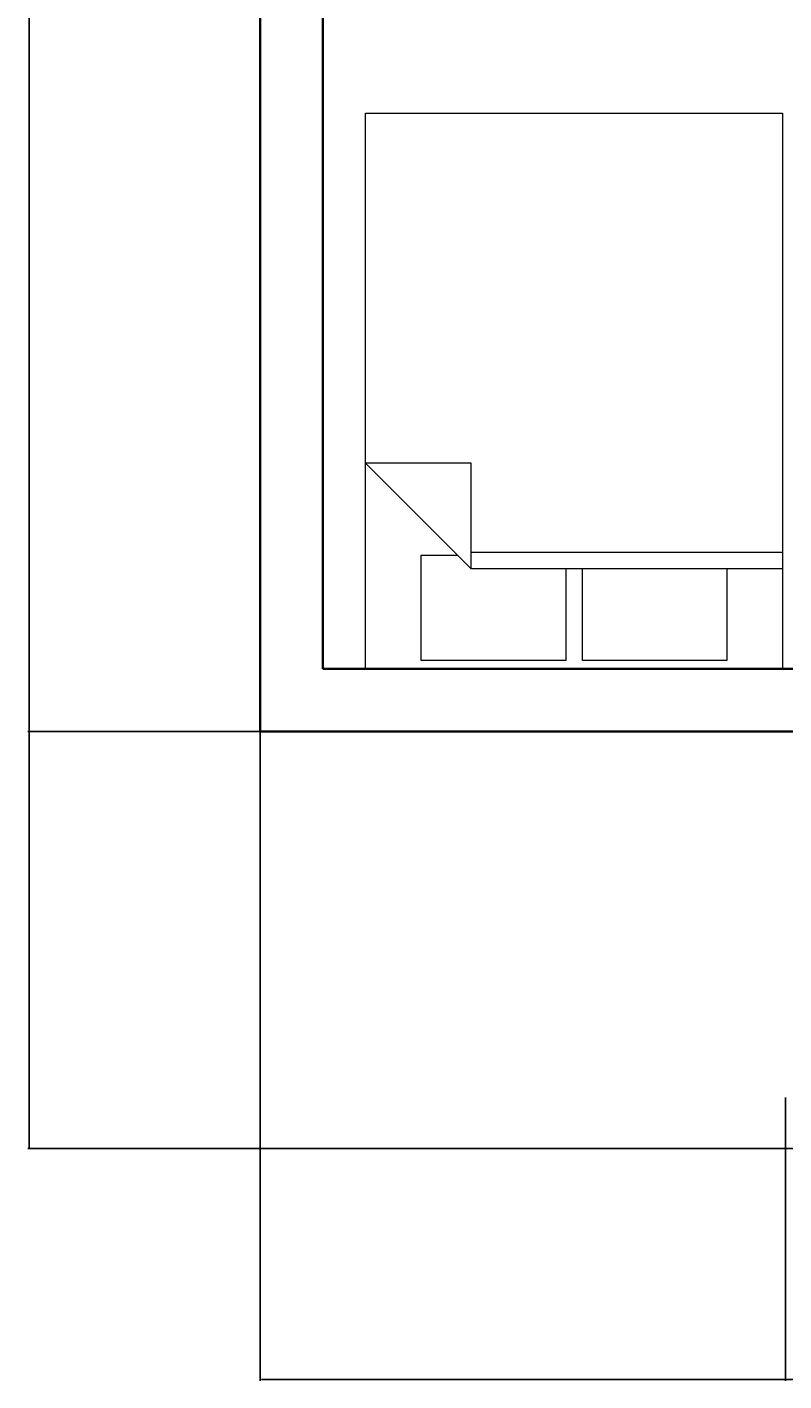
# Model space of a CAD drawing. Units: inches. Extents: x 4159 to 4826, y 299 to 1026.
# Tile 1 of 37: x 4159 to 4268, y 299 to 494. Entities that reach past the tile are written whole.
import ezdxf

# ---------------------------------------------------------------- set-up
doc = ezdxf.new("R2010")
doc.units = ezdxf.units.IN
for name, color, linetype, lineweight in [('A-ANNO-DIMS', 2, 'Continuous', 18), ('A-FURN', 8, 'Continuous', 18), ('A-WALL', 7, 'Continuous', 35)]:
    doc.layers.add(name, color=color, linetype=linetype, lineweight=lineweight)
doc.styles.get("Standard").update_dxf_attribs({"font": 'arial.ttf'})
doc.dimstyles.get("Standard").update_dxf_attribs({"dimtxt": 0.18, "dimasz": 0.18, "dimexe": 0.18, "dimexo": 0.0625, "dimgap": 0.09, "dimtad": 0, "dimtih": 1, "dimtoh": 1, "dimdec": 4, "dimzin": 0, "dimdsep": 46, "dimtxsty": 'Standard', "dimcen": 0.09, "dimadec": 0, "dimazin": 0, "dimtfac": 1, "dimtdec": 4, "dimtofl": 0, "dimtmove": 0, "dimatfit": 3, "dimfxl": 1, "dimtolj": 1, "dimtzin": 0, "dimarcsym": 0})

# ---------------------------------------------------------------- blocks, each defined once
blk = doc.blocks.new('Bed - Queen')
for p, q in [((0, -80.00003), (0, 0)), ((0, 0), (59.99999, 0)), ((59.99999, 0), (59.99999, -80.00003)), ((7.99999, -1.2), (28.79998, -1.2)), ((7.99999, -14.4), (7.99999, -1.2)), ((28.79998, -1.2), (28.79998, -14.4)), ((31.19999, -1.2), (51.99999, -1.2)), ((31.19999, -14.4), (31.19999, -1.2)), ((51.99999, -1.2), (51.99999, -16.4)), ((0, -14.4), (44.8, -14.4)), ((59.99999, -29.6), (44.8, -14.4)), ((44.8, -14.4), (44.8, -29.6)), ((44.8, -16.8), (0, -16.8)), ((51.99999, -16.4), (46.79936, -16.4)), ((44.8, -29.6), (59.99999, -29.6)), ((59.99999, -80.00003), (0, -80.00003))]:
    blk.add_line(p, q)
blk = doc.blocks.new('*D44')
at = {"layer": 'A-ANNO-DIMS', "color": 0, "lineweight": -2, "transparency": 16777216}
for p, q in [((4287.26, 963.09), (4158.88, 963.09)), ((4159.06, 962.91), (4159.06, 647.83)), ((4159.06, 332.38), (4159.06, 647.46)), ((4447.25, 332.2), (4158.88, 332.2))]:
    blk.add_line(p, q, dxfattribs=at)
at = {"layer": 'A-ANNO-DIMS', "color": 0, "transparency": 16777216}
for points in [[(4159.03, 962.91), (4159.09, 962.91), (4159.06, 963.09)], [(4159.03, 332.38), (4159.09, 332.38), (4159.06, 332.2)]]:
    blk.add_solid(points, dxfattribs=at)
at = {"layer": 'Defpoints', "color": 0, "transparency": 16777216}
for p in [(4287.33, 963.09), (4159.06, 332.2), (4447.31, 332.2)]:
    blk.add_point(p, dxfattribs=at)
at = {"layer": 'A-ANNO-DIMS', "color": 0, "transparency": 16777216, "insert": (4159.06, 647.64), "char_height": 0.18, "attachment_point": 5}
blk.add_mtext('\\A1;630.9', dxfattribs=at)
blk = doc.blocks.new('*D46')
at = {"layer": 'A-ANNO-DIMS', "color": 0, "lineweight": -2, "transparency": 16777216}
for p, q in [((4192.31, 392.19), (4192.31, 298.77)), ((4447.31, 332.13), (4447.31, 298.77)), ((4192.49, 298.95), (4319.52, 298.95)), ((4447.13, 298.95), (4320.1, 298.95))]:
    blk.add_line(p, q, dxfattribs=at)
at = {"layer": 'A-ANNO-DIMS', "color": 0, "transparency": 16777216}
for points in [[(4192.49, 298.98), (4192.49, 298.92), (4192.31, 298.95)], [(4447.13, 298.98), (4447.13, 298.92), (4447.31, 298.95)]]:
    blk.add_solid(points, dxfattribs=at)
at = {"layer": 'Defpoints', "color": 0, "transparency": 16777216}
for p in [(4192.31, 392.25), (4447.31, 332.2), (4447.31, 298.95)]:
    blk.add_point(p, dxfattribs=at)
at = {"layer": 'A-ANNO-DIMS', "color": 0, "transparency": 16777216, "insert": (4319.81, 298.95), "char_height": 0.18, "attachment_point": 5}
blk.add_mtext('\\A1;255', dxfattribs=at)
blk = doc.blocks.new('*D50')
at = {"layer": 'A-ANNO-DIMS', "color": 0, "lineweight": -2, "transparency": 16777216}
for p, q in [((4192.31, 392.32), (4192.31, 1025.84)), ((4192.49, 1025.66), (4196.66, 1025.66)), ((4201.13, 1025.66), (4196.96, 1025.66)), ((4201.31, 401.32), (4201.31, 1025.84))]:
    blk.add_line(p, q, dxfattribs=at)
at = {"layer": 'A-ANNO-DIMS', "color": 0, "transparency": 16777216}
for points in [[(4192.49, 1025.69), (4192.49, 1025.63), (4192.31, 1025.66)], [(4201.13, 1025.69), (4201.13, 1025.63), (4201.31, 1025.66)]]:
    blk.add_solid(points, dxfattribs=at)
at = {"layer": 'Defpoints', "color": 0, "transparency": 16777216}
for p in [(4201.31, 1025.66), (4201.31, 401.25), (4192.31, 392.25)]:
    blk.add_point(p, dxfattribs=at)
at = {"layer": 'A-ANNO-DIMS', "color": 0, "transparency": 16777216, "insert": (4196.81, 1025.66), "char_height": 0.18, "attachment_point": 5}
blk.add_mtext('\\A1;9', dxfattribs=at)
blk = doc.blocks.new('*D51')
at = {"layer": 'A-ANNO-DIMS', "color": 0, "lineweight": -2, "transparency": 16777216}
for p, q in [((4201.25, 660.25), (4158.88, 660.25)), ((4159.06, 660.07), (4159.06, 526.44)), ((4159.06, 392.43), (4159.06, 526.07)), ((4192.25, 392.25), (4158.88, 392.25))]:
    blk.add_line(p, q, dxfattribs=at)
at = {"layer": 'A-ANNO-DIMS', "color": 0, "transparency": 16777216}
for points in [[(4159.03, 660.07), (4159.09, 660.07), (4159.06, 660.25)], [(4159.03, 392.43), (4159.09, 392.43), (4159.06, 392.25)]]:
    blk.add_solid(points, dxfattribs=at)
at = {"layer": 'Defpoints', "color": 0, "transparency": 16777216}
for p in [(4159.06, 660.25), (4201.31, 660.25), (4192.31, 392.25)]:
    blk.add_point(p, dxfattribs=at)
at = {"layer": 'A-ANNO-DIMS', "color": 0, "transparency": 16777216, "insert": (4159.06, 526.25), "char_height": 0.18, "attachment_point": 5}
blk.add_mtext('\\A1;268', dxfattribs=at)
blk = doc.blocks.new('*D52')
at = {"layer": 'A-ANNO-DIMS', "color": 0, "lineweight": -2, "transparency": 16777216}
for p, q in [((4192.31, 392.19), (4192.31, 298.77)), ((4267.89, 339.58), (4267.89, 298.77)), ((4192.49, 298.95), (4229.71, 298.95)), ((4267.71, 298.95), (4230.49, 298.95))]:
    blk.add_line(p, q, dxfattribs=at)
at = {"layer": 'A-ANNO-DIMS', "color": 0, "transparency": 16777216}
for points in [[(4192.49, 298.98), (4192.49, 298.92), (4192.31, 298.95)], [(4267.71, 298.98), (4267.71, 298.92), (4267.89, 298.95)]]:
    blk.add_solid(points, dxfattribs=at)
at = {"layer": 'Defpoints', "color": 0, "transparency": 16777216}
for p in [(4192.31, 392.25), (4267.89, 339.64), (4267.89, 298.95)]:
    blk.add_point(p, dxfattribs=at)
at = {"layer": 'A-ANNO-DIMS', "color": 0, "transparency": 16777216, "insert": (4230.1, 298.95), "char_height": 0.18, "attachment_point": 5}
blk.add_mtext('\\A1;75.58', dxfattribs=at)

msp = doc.modelspace()

# ---------------------------------------------------------------- linework, layer by layer
at = {"layer": 'A-WALL'}
for p, q in [((4201.31, 533.254), (4201.31, 401.254)), ((4279.31, 401.254), (4201.31, 401.254)), ((4279.31, 392.254), (4192.31, 392.254))]:
    msp.add_line(p, q, dxfattribs=at)
msp.add_lwpolyline([(4303.31, 903.254), (4192.31, 903.254), (4192.31, 392.254)], dxfattribs=at)

# ---------------------------------------------------------------- block references
at = {"layer": 'A-FURN', "rotation": 180}
msp.add_blockref('Bed - Queen', (4267.473, 401.254), dxfattribs=at)

# ---------------------------------------------------------------- dimensions: what is measured, and where the dimension line sits
at = {"layer": 'A-ANNO-DIMS'}
for base, p2, override, picture, middle in [((4201.31, 1025.662), (4201.31, 401.254), {"dimdec": 0, "dimlfac": 1, "dimrnd": 0, "dimzin": 0, "dimdsep": 46, "dimlunit": 2}, '*D50', (4196.81, 1025.662)), ((4447.31, 298.945), (4447.31, 332.195), {"dimdec": 0, "dimlfac": 1, "dimrnd": 0, "dimzin": 0, "dimdsep": 46, "dimlunit": 2}, '*D46', (4319.81, 298.945)), ((4267.89, 298.945), (4267.89, 339.644), {"dimdec": 2, "dimlfac": 1, "dimrnd": 0, "dimzin": 0, "dimdsep": 46, "dimlunit": 2}, '*D52', (4230.1, 298.945))]:
    dim = msp.add_linear_dim(base=base, p1=(4192.31, 392.254), p2=p2, dimstyle='Standard', override=override, dxfattribs=at)
    dim.commit()
    dim.dimension.update_dxf_attribs({"geometry": picture, "text_midpoint": middle})
for base, p1, p2, override, picture, middle in [((4159.06, 332.195), (4287.326, 963.093), (4447.31, 332.195), {"dimdec": 1, "dimlfac": 1, "dimrnd": 0, "dimzin": 0, "dimdsep": 46, "dimlunit": 2}, '*D44', (4159.06, 647.644)), ((4159.06, 660.254), (4192.31, 392.254), (4201.31, 660.254), {"dimdec": 0, "dimlfac": 1, "dimrnd": 0, "dimzin": 0, "dimdsep": 46, "dimlunit": 2}, '*D51', (4159.06, 526.254))]:
    dim = msp.add_linear_dim(base=base, p1=p1, p2=p2, angle=90, dimstyle='Standard', override=override, dxfattribs=at)
    dim.commit()
    dim.dimension.update_dxf_attribs({"geometry": picture, "text_midpoint": middle})

doc.saveas('drawing.dxf')
